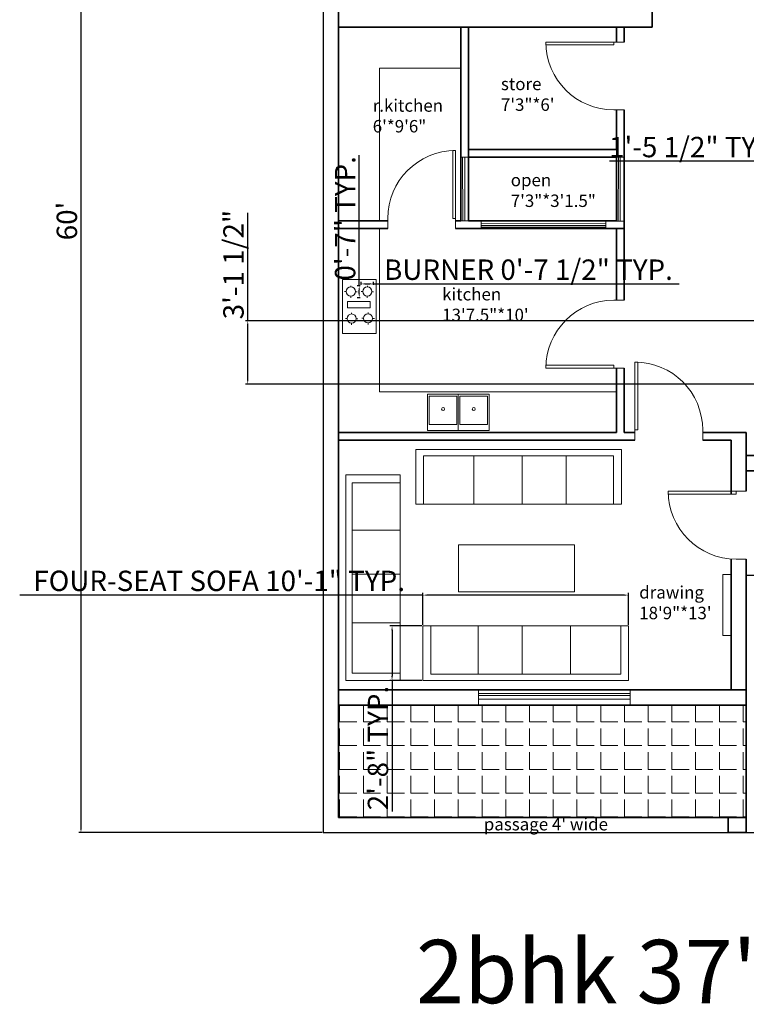
# Model space of a CAD drawing. Units: inches. Extents: x 3067 to 3879, y 3815 to 4813.
# Tile 1 of 3: x 3067 to 3494, y 3815 to 4395. Entities that reach past the tile are written whole.
import ezdxf

# ---------------------------------------------------------------- set-up
doc = ezdxf.new("R2010")
doc.units = ezdxf.units.IN
for name, color, linetype, lineweight in [('A-ANNO-DIMS', 2, 'Continuous', 18), ('A-ANNO-TEXT', 7, 'Continuous', 25), ('A-AREA-IDEN', 7, 'Continuous', 18), ('A-COLS', 7, 'Continuous', 35), ('A-DOOR', 3, 'Continuous', 18), ('A-EQPM', 8, 'Continuous', 18), ('A-FLOR-CASE', 8, 'Continuous', 20), ('A-FLOR-FIXT', 9, 'Continuous', 18), ('A-FLOR-PATT', 252, 'Continuous', 13), ('A-FLOR-STRS', 7, 'Continuous', 25), ('A-FURN', 8, 'Continuous', 18), ('A-GLAZ', 4, 'Continuous', 18), ('A-WALL', 7, 'Continuous', 35), ('C-PROP', 7, 'Continuous', 30)]:
    doc.layers.add(name, color=color, linetype=linetype, lineweight=lineweight)
doc.styles.get("Standard").update_dxf_attribs({"font": 'arial.ttf'})
doc.dimstyles.new('ISO-25', dxfattribs={"dimtxt": 12, "dimasz": 2.5, "dimexe": 1.25, "dimexo": 0.625, "dimtad": 1, "dimdec": 0, "dimlunit": 4, "dimtxsty": 'Standard', "dimcen": 2.5, "dimadec": 0, "dimazin": 0, "dimtfac": 1, "dimtdec": 0, "dimtmove": 0, "dimatfit": 3, "dimfxl": 1, "dimarcsym": 0})

# ---------------------------------------------------------------- blocks, each defined once
blk = doc.blocks.new('*U2')
for p, q in [((0, 0), (0, -6)), ((40, 0), (40, -6))]:
    blk.add_line(p, q)
blk.add_lwpolyline([(0, 0), (0, 40), (1.75, 40), (1.75, 0)], close=True)
blk.add_arc((0, 0), 40, 0, 90)
blk = doc.blocks.new('*D8')
at = {"layer": 'A-ANNO-DIMS', "color": 0, "lineweight": -2, "transparency": 16777216}
for p, q in [((3244.78, 4636.27), (3101.49, 4636.27)), ((3102.74, 4633.77), (3102.74, 3918.77)), ((3244.78, 3916.27), (3101.49, 3916.27))]:
    blk.add_line(p, q, dxfattribs=at)
at = {"layer": 'A-ANNO-DIMS', "color": 0, "lineweight": 100, "transparency": 16777216}
for points in [[(3102.32, 4633.77), (3103.16, 4633.77), (3102.74, 4636.27)], [(3102.32, 3918.77), (3103.16, 3918.77), (3102.74, 3916.27)]]:
    blk.add_solid(points, dxfattribs=at)
at = {"layer": 'Defpoints', "color": 0, "lineweight": 100, "transparency": 16777216}
for p in [(3245.41, 4636.27), (3102.74, 3916.27), (3245.41, 3916.27)]:
    blk.add_point(p, dxfattribs=at)
at = {"layer": 'A-ANNO-DIMS', "color": 0, "transparency": 16777216, "insert": (3095.99, 4276.27), "char_height": 12, "attachment_point": 5, "rotation": 90}
blk.add_mtext("60'", dxfattribs=at)
blk = doc.blocks.new('SOFA-4-SEAT')
for p, q in [((0, 0), (0, 32.05)), ((0, 32.05), (120.99, 32.05)), ((120.99, 32.05), (120.99, 0)), ((34.06, 28.29), (34.06, 0)), ((62.59, 28.29), (62.59, 0)), ((88.47, 28.29), (88.47, 0)), ((4.42, 0), (0, 0)), ((120.99, 0), (116.34, 0))]:
    blk.add_line(p, q)
blk.add_lwpolyline([(4.42, 28.29), (116.34, 28.29), (116.34, 0), (4.42, 0)], close=True)
blk = doc.blocks.new('BURNER')
for p, q in [((3.71, 6.35), (3.71, 7.04)), ((0.98, 3.77), (0, 3.77)), ((3.67, 0.96), (3.67, 0)), ((6.36, 3.54), (7.38, 3.54))]:
    blk.add_line(p, q)
blk.add_circle((3.67, 3.66), 2.69)
blk = doc.blocks.new('GATE-POST')
blk.add_line((10.76, 9), (10.76, 0))
blk.add_lwpolyline([(10.76, 9), (0, 9), (0, 0), (10.76, 0)], close=True)
blk = doc.blocks.new('*D22')
at = {"layer": 'A-ANNO-DIMS', "color": 0, "lineweight": -2, "transparency": 16777216}
for p, q in [((3517.51, 4309.05), (3517.51, 4312.65)), ((3535.11, 4309.05), (3535.11, 4312.65)), ((3517.51, 4311.4), (3413.79, 4311.4)), ((3532.61, 4311.4), (3520.01, 4311.4))]:
    blk.add_line(p, q, dxfattribs=at)
at = {"layer": 'A-ANNO-DIMS', "color": 0, "lineweight": 100, "transparency": 16777216}
for points in [[(3520.01, 4311.82), (3520.01, 4310.99), (3517.51, 4311.4)], [(3532.61, 4311.82), (3532.61, 4310.99), (3535.11, 4311.4)]]:
    blk.add_solid(points, dxfattribs=at)
at = {"layer": 'Defpoints', "color": 0, "lineweight": 100, "transparency": 16777216}
for p in [(3517.51, 4311.4), (3517.51, 4308.43), (3535.11, 4308.43)]:
    blk.add_point(p, dxfattribs=at)
at = {"layer": 'A-ANNO-DIMS', "color": 0, "transparency": 16777216, "insert": (3464.4, 4318.23), "char_height": 12, "attachment_point": 5}
blk.add_mtext('1\'-5 1/2" TYP.', dxfattribs=at)
blk = doc.blocks.new('*D25')
at = {"layer": 'A-ANNO-DIMS', "color": 0, "lineweight": -2, "transparency": 16777216}
for p, q in [((3267.64, 4238.75), (3267.64, 4240.48)), ((3270.14, 4239.23), (3272.52, 4239.23)), ((3275.02, 4238.75), (3275.02, 4240.48)), ((3275.02, 4239.23), (3454.79, 4239.23))]:
    blk.add_line(p, q, dxfattribs=at)
at = {"layer": 'A-ANNO-DIMS', "color": 0, "lineweight": 100, "transparency": 16777216}
for points in [[(3270.14, 4239.65), (3270.14, 4238.82), (3267.64, 4239.23)], [(3272.52, 4239.65), (3272.52, 4238.82), (3275.02, 4239.23)]]:
    blk.add_solid(points, dxfattribs=at)
at = {"layer": 'Defpoints', "color": 0, "lineweight": 100, "transparency": 16777216}
for p in [(3267.64, 4238.13), (3275.02, 4239.23), (3275.02, 4238.13)]:
    blk.add_point(p, dxfattribs=at)
at = {"layer": 'A-ANNO-DIMS', "color": 0, "transparency": 16777216, "insert": (3366.16, 4246.06), "char_height": 12, "attachment_point": 5}
blk.add_mtext('BURNER 0\'-7 1/2" TYP.', dxfattribs=at)
blk = doc.blocks.new('*D26')
at = {"layer": 'A-ANNO-DIMS', "color": 0, "lineweight": -2, "transparency": 16777216}
for p, q in [((3266.53, 4238.13), (3266.53, 4315.02)), ((3267.02, 4238.13), (3265.28, 4238.13)), ((3267.02, 4231.09), (3265.28, 4231.09)), ((3266.53, 4233.59), (3266.53, 4235.63))]:
    blk.add_line(p, q, dxfattribs=at)
at = {"layer": 'A-ANNO-DIMS', "color": 0, "lineweight": 100, "transparency": 16777216}
for points in [[(3266.12, 4235.63), (3266.95, 4235.63), (3266.53, 4238.13)], [(3266.12, 4233.59), (3266.95, 4233.59), (3266.53, 4231.09)]]:
    blk.add_solid(points, dxfattribs=at)
at = {"layer": 'Defpoints', "color": 0, "lineweight": 100, "transparency": 16777216}
for p in [(3266.53, 4238.13), (3267.64, 4238.13), (3267.64, 4231.09)]:
    blk.add_point(p, dxfattribs=at)
at = {"layer": 'A-ANNO-DIMS', "color": 0, "transparency": 16777216, "insert": (3259.78, 4277.83), "char_height": 12, "attachment_point": 5, "rotation": 90}
blk.add_mtext('0\'-7" TYP.', dxfattribs=at)
blk = doc.blocks.new('*D27')
at = {"layer": 'A-ANNO-DIMS', "color": 0, "lineweight": -2, "transparency": 16777216}
for p, q in [((3304.02, 4038.55), (3304.02, 4057.33)), ((3425.01, 4038.55), (3425.01, 4057.33)), ((3304.02, 4056.08), (3066.67, 4056.08)), ((3422.51, 4056.08), (3306.52, 4056.08))]:
    blk.add_line(p, q, dxfattribs=at)
at = {"layer": 'A-ANNO-DIMS', "color": 0, "lineweight": 100, "transparency": 16777216}
for points in [[(3306.52, 4056.49), (3306.52, 4055.66), (3304.02, 4056.08)], [(3422.51, 4056.49), (3422.51, 4055.66), (3425.01, 4056.08)]]:
    blk.add_solid(points, dxfattribs=at)
at = {"layer": 'Defpoints', "color": 0, "lineweight": 100, "transparency": 16777216}
for p in [(3304.02, 4056.08), (3304.02, 4037.93), (3425.01, 4037.93)]:
    blk.add_point(p, dxfattribs=at)
at = {"layer": 'A-ANNO-DIMS', "color": 0, "transparency": 16777216, "insert": (3184.09, 4062.91), "char_height": 12, "attachment_point": 5}
blk.add_mtext('FOUR-SEAT SOFA 10\'-1" TYP.', dxfattribs=at)
blk = doc.blocks.new('*D28')
at = {"layer": 'A-ANNO-DIMS', "color": 0, "lineweight": -2, "transparency": 16777216}
for p, q in [((3303.4, 4037.93), (3284.62, 4037.93)), ((3285.87, 4035.43), (3285.87, 4008.38)), ((3303.4, 4005.88), (3284.62, 4005.88)), ((3285.87, 4005.88), (3285.87, 3928.78))]:
    blk.add_line(p, q, dxfattribs=at)
at = {"layer": 'A-ANNO-DIMS', "color": 0, "lineweight": 100, "transparency": 16777216}
for points in [[(3285.46, 4035.43), (3286.29, 4035.43), (3285.87, 4037.93)], [(3285.46, 4008.38), (3286.29, 4008.38), (3285.87, 4005.88)]]:
    blk.add_solid(points, dxfattribs=at)
at = {"layer": 'Defpoints', "color": 0, "lineweight": 100, "transparency": 16777216}
for p in [(3304.02, 4037.93), (3285.87, 4005.88), (3304.02, 4005.88)]:
    blk.add_point(p, dxfattribs=at)
at = {"layer": 'A-ANNO-DIMS', "color": 0, "transparency": 16777216, "insert": (3279.12, 3966.08), "char_height": 12, "attachment_point": 5, "rotation": 90}
blk.add_mtext('2\'-8" TYP.', dxfattribs=at)
blk = doc.blocks.new('*D48')
at = {"layer": 'A-ANNO-DIMS', "color": 0, "lineweight": -2, "transparency": 16777216}
for p, q in [((3200.91, 4217.55), (3200.91, 4281.15)), ((3571.24, 4217.55), (3199.66, 4217.55)), ((3200.91, 4182.77), (3200.91, 4215.05)), ((3571.24, 4180.27), (3199.66, 4180.27))]:
    blk.add_line(p, q, dxfattribs=at)
at = {"layer": 'A-ANNO-DIMS', "color": 0, "lineweight": 100, "transparency": 16777216}
for points in [[(3200.49, 4215.05), (3201.32, 4215.05), (3200.91, 4217.55)], [(3200.49, 4182.77), (3201.32, 4182.77), (3200.91, 4180.27)]]:
    blk.add_solid(points, dxfattribs=at)
at = {"layer": 'Defpoints', "color": 0, "lineweight": 100, "transparency": 16777216}
for p in [(3200.91, 4217.55), (3571.86, 4217.55), (3571.86, 4180.27)]:
    blk.add_point(p, dxfattribs=at)
at = {"layer": 'A-ANNO-DIMS', "color": 0, "transparency": 16777216, "insert": (3194.07, 4250.6), "char_height": 12, "attachment_point": 5, "rotation": 90}
blk.add_mtext('3\'-1 1/2"', dxfattribs=at)

msp = doc.modelspace()

# ---------------------------------------------------------------- hatches: boundary and pattern name
at = {"layer": 'A-FLOR-PATT'}
h = msp.add_hatch(dxfattribs=at)
h.set_pattern_fill('ANGLE', color=256, scale=2)
h.set_pattern_definition([(0, (0, 0), (0, 13.97), [10.16, -3.81]), (90, (0, 0), (-13.97, 9e-16), [10.16, -3.81])])
h.paths.add_polyline_path([(3494.41, 3991.27), (3489.91, 3991.27), (3479.41, 3991.27), (3254.41, 3991.27), (3254.41, 3925.27), (3494.41, 3925.27)])

# ---------------------------------------------------------------- linework, layer by layer
at = {"layer": 'A-EQPM'}
for points in [[(3256.67, 4241.9), (3276.45, 4241.9), (3276.45, 4210.15), (3256.67, 4210.15)], [(3259.65, 4228.89), (3273.07, 4228.89), (3273.07, 4225.08), (3259.65, 4225.08)], [(3485.41, 4068.23), (3480.5, 4068.23), (3480.5, 4032.32), (3485.41, 4032.32)]]:
    msp.add_lwpolyline(points, close=True, dxfattribs=at)
at = {"layer": 'A-FLOR-CASE'}
for p, q in [((3326.41, 4390.27), (3326.41, 4366.27)), ((3278.41, 4276.27), (3278.41, 4366.27)), ((3326.41, 4366.27), (3278.41, 4366.27)), ((3254.41, 4271.77), (3278.41, 4271.77)), ((3278.41, 4271.77), (3278.41, 4175.77)), ((3417.91, 4175.77), (3278.41, 4175.77)), ((3417.91, 4151.77), (3417.91, 4175.77))]:
    msp.add_line(p, q, dxfattribs=at)
at = {"layer": 'A-FLOR-FIXT'}
msp.add_line((3324.86, 4152.96), (3324.86, 4174.27), dxfattribs=at)
for points in [[(3306.64, 4174.27), (3343.08, 4174.27), (3343.08, 4152.96), (3306.64, 4152.96)], [(3307.74, 4156.48), (3323.97, 4156.48), (3323.97, 4173.08), (3307.74, 4173.08)], [(3325.83, 4156.48), (3342.07, 4156.48), (3342.07, 4173.08), (3325.83, 4173.08)]]:
    msp.add_lwpolyline(points, close=True, dxfattribs=at)
for centre in [(3315.94, 4165.6), (3333.98, 4165.6)]:
    msp.add_circle(centre, 0.875, dxfattribs=at)
at = {"layer": 'A-FLOR-STRS'}
msp.add_line((3494.41, 4067.77), (3514.9, 4067.77), dxfattribs=at)
at = {"layer": 'A-FURN'}
msp.add_lwpolyline([(3324.92, 4085.61), (3393.35, 4085.61), (3393.35, 4057.98), (3324.92, 4057.98)], close=True, dxfattribs=at)
at = {"layer": 'A-GLAZ'}
for p, q in [((3327.45, 4276.27), (3327.39, 4313.77)), ((3328.66, 4276.27), (3328.66, 4313.77)), ((3419.26, 4313.77), (3419.03, 4276.19)), ((3420.16, 4313.77), (3420.16, 4276.19)), ((3338.41, 4274.8), (3411.79, 4274.95)), ((3338.41, 4273.69), (3411.79, 4273.69)), ((3338.41, 4272.71), (3411.79, 4272.71)), ((3336.85, 3998.18), (3426, 3998.18)), ((3336.85, 3996.99), (3426, 3996.99)), ((3336.85, 3994.75), (3426, 3994.75))]:
    msp.add_line(p, q, dxfattribs=at)
for points in [[(3326.41, 4276.27), (3330.91, 4276.27), (3330.91, 4313.77), (3326.41, 4313.77)], [(3417.91, 4313.77), (3422.41, 4313.77), (3422.41, 4276.19), (3417.91, 4276.19)], [(3338.41, 4276.27), (3411.79, 4276.27), (3411.79, 4271.77), (3338.41, 4271.77)], [(3336.85, 4000.27), (3426, 4000.27), (3426, 3991.27), (3336.85, 3991.27)]]:
    msp.add_lwpolyline(points, close=True, dxfattribs=at)
at = {"layer": 'A-WALL'}
for p, q in [((3438.91, 4390.27), (3438.91, 4400.62)), ((3254.41, 4390.27), (3438.91, 4390.27)), ((3254.41, 4390.27), (3254.41, 4276.27)), ((3326.41, 4276.27), (3326.41, 4390.27)), ((3330.91, 4276.27), (3330.91, 4390.27)), ((3330.91, 4390.27), (3417.91, 4390.27)), ((3417.91, 4390.27), (3417.91, 4381.61)), ((3422.41, 4390.27), (3422.41, 4381.61)), ((3417.91, 4341.61), (3417.91, 4318.27)), ((3422.41, 4341.61), (3422.41, 4313.77)), ((3417.91, 4318.27), (3417.91, 4324.48)), ((3417.91, 4318.27), (3330.91, 4318.27)), ((3417.91, 4313.77), (3330.91, 4313.77)), ((3330.91, 4313.77), (3330.91, 4276.27)), ((3417.91, 4276.27), (3417.91, 4313.77)), ((3422.41, 4313.77), (3422.41, 4271.77)), ((3254.41, 4276.27), (3283.31, 4276.27)), ((3254.41, 4271.77), (3283.31, 4271.77)), ((3254.41, 4271.77), (3254.41, 4151.77)), ((3323.31, 4276.27), (3326.41, 4276.27)), ((3323.31, 4271.77), (3330.91, 4271.77)), ((3330.91, 4276.27), (3417.91, 4276.27)), ((3330.91, 4271.77), (3422.41, 4271.77)), ((3417.91, 4229.61), (3417.91, 4271.77)), ((3422.41, 4229.61), (3422.41, 4271.77)), ((3417.91, 4151.77), (3417.91, 4189.61)), ((3422.41, 4151.77), (3422.41, 4189.61)), ((3254.41, 4151.77), (3417.91, 4151.77)), ((3422.41, 4151.77), (3428.73, 4151.77)), ((3468.73, 4151.77), (3494.41, 4151.77)), ((3494.41, 4151.77), (3494.41, 4120.22)), ((3254.41, 4147.27), (3422.41, 4147.27)), ((3254.41, 4147.27), (3254.41, 3991.27)), ((3422.41, 4147.27), (3428.73, 4147.27)), ((3468.73, 4147.27), (3485.41, 4147.27)), ((3485.41, 4147.27), (3485.41, 4129.36)), ((3485.41, 4138.27), (3485.41, 4115.54)), ((3519.03, 4138.27), (3494.41, 4138.27)), ((3494.41, 4129.27), (3494.41, 4117.29)), ((3517.72, 4129.27), (3494.41, 4129.27)), ((3485.41, 4077.4), (3485.41, 4000.27)), ((3494.41, 4077.29), (3494.41, 3925.27)), ((3254.41, 4000.27), (3479.41, 4000.27)), ((3479.41, 4000.27), (3489.91, 4000.27)), ((3489.91, 4000.27), (3494.41, 4000.27)), ((3254.41, 3991.27), (3479.41, 3991.27)), ((3479.41, 3991.27), (3489.91, 3991.27)), ((3489.91, 3991.27), (3494.41, 3991.27))]:
    msp.add_line(p, q, dxfattribs=at)
msp.add_lwpolyline([(3686.41, 4567.27), (3686.41, 4627.27), (3254.41, 4627.27), (3254.41, 3925.27), (3494.41, 3925.27)], dxfattribs=at)
at = {"layer": 'C-PROP'}
msp.add_lwpolyline([(3245.41, 3916.27), (3695.41, 3916.27), (3695.41, 4636.27), (3245.41, 4636.27)], close=True, dxfattribs=at)

# ---------------------------------------------------------------- block references
at = {"layer": 'A-COLS'}
msp.add_blockref('GATE-POST', (3483.64, 3916.27), dxfattribs=at)
at = {"layer": 'A-DOOR', "xscale": -1, "rotation": 90}
for p in [(3416.41, 4381.61), (3488.41, 4117.29)]:
    msp.add_blockref('*U2', p, dxfattribs=at)
at = {"layer": 'A-DOOR', "xscale": -1}
msp.add_blockref('*U2', (3323.31, 4277.77), dxfattribs=at)
at = {"layer": 'A-DOOR', "rotation": 90}
msp.add_blockref('*U2', (3416.41, 4189.61), dxfattribs=at)
at = {"layer": 'A-DOOR'}
msp.add_blockref('*U2', (3428.73, 4153.27), dxfattribs=at)
at = {"layer": 'A-EQPM'}
for p in [(3257.95, 4231.09), (3267.64, 4231.09), (3258.37, 4215.19), (3268.06, 4215.32)]:
    msp.add_blockref('BURNER', p, dxfattribs=at)
at = {"layer": 'A-FURN'}
msp.add_blockref('SOFA-4-SEAT', (3299.94, 4109.69), dxfattribs=at)
for p, rotation in [((3290.66, 4005.79), 90.00000000000055), ((3425.01, 4037.93), 180)]:
    msp.add_blockref('SOFA-4-SEAT', p, dxfattribs=dict(at, rotation=rotation))

# ---------------------------------------------------------------- texts
at = {"layer": 'A-ANNO-TEXT', "insert": (3299.99, 3853.16), "char_height": 37.2582, "attachment_point": 1}
msp.add_mtext_dynamic_manual_height_columns('2bhk 37\'6"*60\'', width=1373.908, gutter_width=186.29, heights=[0], dxfattribs=at)
at = {"layer": 'A-AREA-IDEN', "attachment_point": 1}
for s, insert, char_height in [('store\\P7\'3"*6\'', (3349.96, 4360.58), 7.308), ('r.kitchen\\P6\'*9\'6"', (3274.49, 4347.88), 7.308), ('open\\P7\'3"*3\'1.5"', (3355.74, 4304.02), 7.3083), ('kitchen\\P13\'7.5"*10\'', (3315.37, 4236.85), 7.3083), ('drawing\\P18\'9"*13\'', (3431.36, 4061.39), 7.308), ("passage 4' wide", (3339.87, 3924.91), 7.3083)]:
    msp.add_mtext_dynamic_manual_height_columns(s, width=269.495, gutter_width=36.54, heights=[0], dxfattribs=dict(at, insert=insert, char_height=char_height))

# ---------------------------------------------------------------- dimensions: what is measured, and where the dimension line sits
at = {"layer": 'A-ANNO-DIMS'}
for base, p1, p2, override, picture, middle in [((3102.74, 3916.27), (3245.41, 4636.27), (3245.41, 3916.27), {"dimclrd": 0, "dimclre": 0, "dimclrt": 0}, '*D8', (3095.99, 4276.27)), ((3200.91, 4217.55), (3571.86, 4180.27), (3571.86, 4217.55), {"dimdec": 1, "dimlfac": 1, "dimrnd": 0, "dimzin": 1, "dimdsep": 46, "dimlunit": 4, "dimfrac": 2}, '*D48', (3194.07, 4250.6))]:
    dim = msp.add_linear_dim(base=base, p1=p1, p2=p2, angle=90, dimstyle='ISO-25', override=override, dxfattribs=at)
    dim.commit()
    dim.dimension.update_dxf_attribs({"geometry": picture, "text_midpoint": middle})
for base, p1, p2, angle, text, picture, middle in [((3517.51, 4311.4), (3535.11, 4308.43), (3517.51, 4308.43), 180, '<> TYP.', '*D22', (3464.4, 4318.23)), ((3266.53, 4238.13), (3267.64, 4231.09), (3267.64, 4238.13), 90, '<> TYP.', '*D26', (3259.78, 4277.83)), ((3304.02, 4056.08), (3425.01, 4037.93), (3304.02, 4037.93), 180, 'FOUR-SEAT SOFA <> TYP.', '*D27', (3184.09, 4062.91)), ((3285.8748, 4005.883), (3304.0225, 4037.9284), (3304.0225, 4005.883), 270, '<> TYP.', '*D28', (3279.1229, 3966.0827))]:
    dim = msp.add_linear_dim(base=base, p1=p1, p2=p2, angle=angle, text=text, dimstyle='ISO-25', override={"dimdec": 1, "dimlfac": 1, "dimrnd": 0, "dimzin": 1, "dimdsep": 46, "dimlunit": 4, "dimfrac": 2}, dxfattribs=at)
    dim.commit()
    dim.dimension.update_dxf_attribs({"geometry": picture, "text_midpoint": middle})
dim = msp.add_linear_dim(base=(3275.02, 4239.23), p1=(3267.64, 4238.13), p2=(3275.02, 4238.13), text='BURNER <> TYP.', dimstyle='ISO-25', override={"dimdec": 1, "dimlfac": 1, "dimrnd": 0, "dimzin": 1, "dimdsep": 46, "dimlunit": 4, "dimfrac": 2}, dxfattribs=at)
dim.commit()
dim.dimension.update_dxf_attribs({"geometry": '*D25', "text_midpoint": (3366.16, 4246.06)})

doc.saveas('drawing.dxf')
